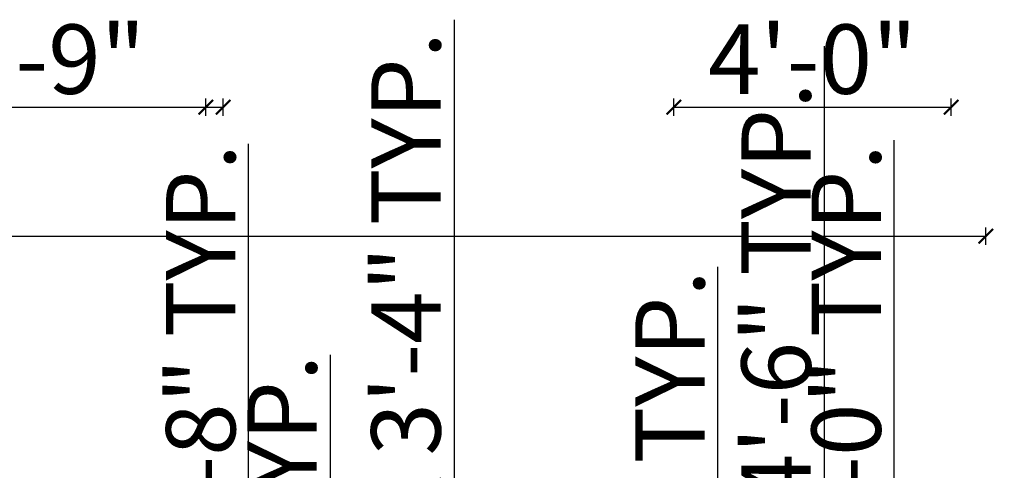
# Model space of a CAD drawing. Units: inches. Extents: x 375 to 1122, y 27 to 1069.
# Tile 154 of 155: x 819 to 989, y 991 to 1069. Entities that reach past the tile are written whole.
import ezdxf

# ---------------------------------------------------------------- set-up
doc = ezdxf.new("R2010")
doc.units = ezdxf.units.IN
doc.layers.add('A-ANNO-DIMS', color=2, linetype='Continuous', lineweight=18)
doc.styles.get("Standard").update_dxf_attribs({"font": 'arial.ttf'})
doc.dimstyles.new('ISO-25', dxfattribs={"dimtxt": 12, "dimasz": 2.5, "dimexe": 1.5, "dimexo": 1.5, "dimtad": 1, "dimdec": 1, "dimlunit": 3, "dimtxsty": 'Standard', "dimblk": 'ARCHTICK', "dimcen": 2.5, "dimadec": 0, "dimazin": 0, "dimtfac": 1, "dimtdec": 1, "dimtmove": 0, "dimatfit": 3, "dimfxl": 1.5, "dimfxlon": 1, "dimarcsym": 0})

# ---------------------------------------------------------------- blocks, each defined once
blk = doc.blocks.new('_ArchTick')
at = {"color": 0, "linetype": 'ByBlock', "const_width": 0.15}
blk.add_lwpolyline([(-0.5, -0.5), (0.5, 0.5)], dxfattribs=at)
blk = doc.blocks.new('*D27')
at = {"layer": 'A-ANNO-DIMS', "color": 0, "lineweight": -2, "transparency": 16777216}
for p, q in [((444.51, 1030.21), (444.51, 1033.21)), ((986.01, 1030.21), (986.01, 1033.21)), ((444.51, 1031.71), (986.01, 1031.71))]:
    blk.add_line(p, q, dxfattribs=at)
at = {"layer": 'Defpoints', "color": 0, "transparency": 16777216}
for p in [(986.01, 1031.71), (444.51, 982.53), (986.01, 982.53)]:
    blk.add_point(p, dxfattribs=at)
at = {"layer": 'A-ANNO-DIMS', "color": 0, "lineweight": -2, "transparency": 16777216, "xscale": 2.5, "yscale": 2.5, "zscale": 2.5, "rotation": 180}
blk.add_blockref('_ArchTick', (444.51, 1031.71), dxfattribs=at)
at = {"layer": 'A-ANNO-DIMS', "color": 0, "lineweight": -2, "transparency": 16777216, "xscale": 2.5, "yscale": 2.5, "zscale": 2.5}
blk.add_blockref('_ArchTick', (986.01, 1031.71), dxfattribs=at)
at = {"layer": 'A-ANNO-DIMS', "color": 0, "transparency": 16777216, "insert": (715.26, 1038.46), "char_height": 12, "attachment_point": 5}
blk.add_mtext('45\'-1.5"', dxfattribs=at)
blk = doc.blocks.new('*D62')
at = {"layer": 'A-ANNO-DIMS', "color": 0, "lineweight": -2, "transparency": 16777216}
for p, q in [((872.61, 898.16), (872.61, 1011.21)), ((871.11, 898.16), (874.11, 898.16)), ((872.61, 874.53), (872.61, 898.16)), ((871.11, 874.53), (874.11, 874.53))]:
    blk.add_line(p, q, dxfattribs=at)
at = {"layer": 'Defpoints', "color": 0, "transparency": 16777216}
for p in [(869.01, 898.16), (872.61, 898.16), (869.01, 874.53)]:
    blk.add_point(p, dxfattribs=at)
at = {"layer": 'A-ANNO-DIMS', "color": 0, "lineweight": -2, "transparency": 16777216, "xscale": 2.5, "yscale": 2.5, "zscale": 2.5}
for p, rotation in [((872.61, 898.16), 90), ((872.61, 874.53), 270)]:
    blk.add_blockref('_ArchTick', p, dxfattribs=dict(at, rotation=rotation))
at = {"layer": 'A-ANNO-DIMS', "color": 0, "transparency": 16777216, "insert": (865.78, 955.93), "char_height": 12, "attachment_point": 5, "rotation": 90}
blk.add_mtext('1\'-11 1/2" TYP.', dxfattribs=at)
blk = doc.blocks.new('*D63')
at = {"layer": 'A-ANNO-DIMS', "color": 0, "lineweight": -2, "transparency": 16777216}
for p, q in [((894.04, 948.53), (894.04, 1069.15)), ((895.54, 948.53), (892.54, 948.53)), ((894.04, 908.53), (894.04, 948.53)), ((895.54, 908.53), (892.54, 908.53))]:
    blk.add_line(p, q, dxfattribs=at)
at = {"layer": 'Defpoints', "color": 0, "transparency": 16777216}
for p in [(894.04, 948.53), (900.04, 948.53), (900.04, 908.53)]:
    blk.add_point(p, dxfattribs=at)
at = {"layer": 'A-ANNO-DIMS', "color": 0, "lineweight": -2, "transparency": 16777216, "xscale": 2.5, "yscale": 2.5, "zscale": 2.5}
for p, rotation in [((894.04, 948.53), 90), ((894.04, 908.53), 270)]:
    blk.add_blockref('_ArchTick', p, dxfattribs=dict(at, rotation=rotation))
at = {"layer": 'A-ANNO-DIMS', "color": 0, "transparency": 16777216, "insert": (887.21, 1010.09), "char_height": 12, "attachment_point": 5, "rotation": 90}
blk.add_mtext('SINK 3\'-4" TYP.', dxfattribs=at)
blk = doc.blocks.new('*D66')
at = {"layer": 'A-ANNO-DIMS', "color": 0, "lineweight": -2, "transparency": 16777216}
for p, q in [((970.15, 971.21), (970.15, 1048.31)), ((968.65, 971.21), (971.65, 971.21)), ((970.15, 947.21), (970.15, 971.21)), ((968.65, 947.21), (971.65, 947.21))]:
    blk.add_line(p, q, dxfattribs=at)
at = {"layer": 'Defpoints', "color": 0, "transparency": 16777216}
for p in [(966.55, 971.21), (970.15, 971.21), (966.55, 947.21)]:
    blk.add_point(p, dxfattribs=at)
at = {"layer": 'A-ANNO-DIMS', "color": 0, "lineweight": -2, "transparency": 16777216, "xscale": 2.5, "yscale": 2.5, "zscale": 2.5}
for p, rotation in [((970.15, 971.21), 90), ((970.15, 947.21), 270)]:
    blk.add_blockref('_ArchTick', p, dxfattribs=dict(at, rotation=rotation))
at = {"layer": 'A-ANNO-DIMS', "color": 0, "transparency": 16777216, "insert": (963.4, 1011.01), "char_height": 12, "attachment_point": 5, "rotation": 90}
blk.add_mtext('2\'-0" TYP.', dxfattribs=at)
blk = doc.blocks.new('*D68')
at = {"layer": 'A-ANNO-DIMS', "color": 0, "lineweight": -2, "transparency": 16777216}
for p, q in [((858.44, 971.91), (858.44, 1047.67)), ((856.94, 971.91), (859.94, 971.91)), ((858.44, 951.91), (858.44, 971.91)), ((856.94, 951.91), (859.94, 951.91))]:
    blk.add_line(p, q, dxfattribs=at)
at = {"layer": 'Defpoints', "color": 0, "transparency": 16777216}
for p in [(853.33, 971.91), (858.44, 971.91), (853.33, 951.91)]:
    blk.add_point(p, dxfattribs=at)
at = {"layer": 'A-ANNO-DIMS', "color": 0, "lineweight": -2, "transparency": 16777216, "xscale": 2.5, "yscale": 2.5, "zscale": 2.5}
for p, rotation in [((858.44, 971.91), 90), ((858.44, 951.91), 270)]:
    blk.add_blockref('_ArchTick', p, dxfattribs=dict(at, rotation=rotation))
at = {"layer": 'A-ANNO-DIMS', "color": 0, "transparency": 16777216, "insert": (851.69, 1011.04), "char_height": 12, "attachment_point": 5, "rotation": 90}
blk.add_mtext('1\'-8" TYP.', dxfattribs=at)
blk = doc.blocks.new('*D75')
at = {"layer": 'A-ANNO-DIMS', "color": 0, "lineweight": -2, "transparency": 16777216}
for p, q in [((958.11, 868.53), (958.11, 1064.59)), ((956.61, 868.53), (959.61, 868.53)), ((958.11, 814.53), (958.11, 868.53)), ((956.61, 814.53), (959.61, 814.53))]:
    blk.add_line(p, q, dxfattribs=at)
at = {"layer": 'Defpoints', "color": 0, "transparency": 16777216}
for p in [(950.01, 868.53), (958.11, 868.53), (950.01, 814.53)]:
    blk.add_point(p, dxfattribs=at)
at = {"layer": 'A-ANNO-DIMS', "color": 0, "lineweight": -2, "transparency": 16777216, "xscale": 2.5, "yscale": 2.5, "zscale": 2.5}
for p, rotation in [((958.11, 868.53), 90), ((958.11, 814.53), 270)]:
    blk.add_blockref('_ArchTick', p, dxfattribs=dict(at, rotation=rotation))
at = {"layer": 'A-ANNO-DIMS', "color": 0, "transparency": 16777216, "insert": (951.27, 967.81), "char_height": 12, "attachment_point": 5, "rotation": 90}
blk.add_mtext('SHOWER PAN 4\'-6" TYP.', dxfattribs=at)
blk = doc.blocks.new('*D78')
at = {"layer": 'A-ANNO-DIMS', "color": 0, "lineweight": -2, "transparency": 16777216}
for p, q in [((939.66, 949.53), (939.66, 1026.42)), ((938.16, 949.53), (941.16, 949.53)), ((939.66, 907.53), (939.66, 949.53)), ((938.16, 907.53), (941.16, 907.53))]:
    blk.add_line(p, q, dxfattribs=at)
at = {"layer": 'Defpoints', "color": 0, "transparency": 16777216}
for p in [(923.01, 949.53), (939.66, 949.53), (923.01, 907.53)]:
    blk.add_point(p, dxfattribs=at)
at = {"layer": 'A-ANNO-DIMS', "color": 0, "lineweight": -2, "transparency": 16777216, "xscale": 2.5, "yscale": 2.5, "zscale": 2.5}
for p, rotation in [((939.66, 949.53), 90), ((939.66, 907.53), 270)]:
    blk.add_blockref('_ArchTick', p, dxfattribs=dict(at, rotation=rotation))
at = {"layer": 'A-ANNO-DIMS', "color": 0, "transparency": 16777216, "insert": (932.9, 989.22), "char_height": 12, "attachment_point": 5, "rotation": 90}
blk.add_mtext('3\'-6" TYP.', dxfattribs=at)
blk = doc.blocks.new('*D83')
at = {"layer": 'A-ANNO-DIMS', "color": 0, "lineweight": -2, "transparency": 16777216}
for p, q in [((932.01, 1052.53), (932.01, 1055.53)), ((980.01, 1052.53), (980.01, 1055.53)), ((932.01, 1054.03), (980.01, 1054.03))]:
    blk.add_line(p, q, dxfattribs=at)
at = {"layer": 'Defpoints', "color": 0, "transparency": 16777216}
for p in [(980.01, 1054.03), (932.01, 973.53), (980.01, 973.53)]:
    blk.add_point(p, dxfattribs=at)
at = {"layer": 'A-ANNO-DIMS', "color": 0, "lineweight": -2, "transparency": 16777216, "xscale": 2.5, "yscale": 2.5, "zscale": 2.5, "rotation": 180}
blk.add_blockref('_ArchTick', (932.01, 1054.03), dxfattribs=at)
at = {"layer": 'A-ANNO-DIMS', "color": 0, "lineweight": -2, "transparency": 16777216, "xscale": 2.5, "yscale": 2.5, "zscale": 2.5}
blk.add_blockref('_ArchTick', (980.01, 1054.03), dxfattribs=at)
at = {"layer": 'A-ANNO-DIMS', "color": 0, "transparency": 16777216, "insert": (956.01, 1060.78), "char_height": 12, "attachment_point": 5}
blk.add_mtext('4\'-0"', dxfattribs=at)
blk = doc.blocks.new('*D88')
at = {"layer": 'A-ANNO-DIMS', "color": 0, "lineweight": -2, "transparency": 16777216}
for p, q in [((731.01, 1052.53), (731.01, 1055.53)), ((854.01, 1052.53), (854.01, 1055.53)), ((731.01, 1054.03), (854.01, 1054.03))]:
    blk.add_line(p, q, dxfattribs=at)
at = {"layer": 'Defpoints', "color": 0, "transparency": 16777216}
for p in [(854.01, 1054.03), (731.01, 502.53), (854.01, 502.53)]:
    blk.add_point(p, dxfattribs=at)
at = {"layer": 'A-ANNO-DIMS', "color": 0, "lineweight": -2, "transparency": 16777216, "xscale": 2.5, "yscale": 2.5, "zscale": 2.5, "rotation": 180}
blk.add_blockref('_ArchTick', (731.01, 1054.03), dxfattribs=at)
at = {"layer": 'A-ANNO-DIMS', "color": 0, "lineweight": -2, "transparency": 16777216, "xscale": 2.5, "yscale": 2.5, "zscale": 2.5}
blk.add_blockref('_ArchTick', (854.01, 1054.03), dxfattribs=at)
at = {"layer": 'A-ANNO-DIMS', "color": 0, "transparency": 16777216, "insert": (792.51, 1060.78), "char_height": 12, "attachment_point": 5}
blk.add_mtext('10\'-3"', dxfattribs=at)
blk = doc.blocks.new('*D96')
at = {"layer": 'A-ANNO-DIMS', "color": 0, "lineweight": -2, "transparency": 16777216}
for p, q in [((794.01, 1052.53), (794.01, 1055.53)), ((851.01, 1052.53), (851.01, 1055.53)), ((794.01, 1054.03), (851.01, 1054.03))]:
    blk.add_line(p, q, dxfattribs=at)
at = {"layer": 'Defpoints', "color": 0, "transparency": 16777216}
for p in [(851.01, 1054.03), (794.01, 973.53), (851.01, 973.53)]:
    blk.add_point(p, dxfattribs=at)
at = {"layer": 'A-ANNO-DIMS', "color": 0, "lineweight": -2, "transparency": 16777216, "xscale": 2.5, "yscale": 2.5, "zscale": 2.5, "rotation": 180}
blk.add_blockref('_ArchTick', (794.01, 1054.03), dxfattribs=at)
at = {"layer": 'A-ANNO-DIMS', "color": 0, "lineweight": -2, "transparency": 16777216, "xscale": 2.5, "yscale": 2.5, "zscale": 2.5}
blk.add_blockref('_ArchTick', (851.01, 1054.03), dxfattribs=at)
at = {"layer": 'A-ANNO-DIMS', "color": 0, "transparency": 16777216, "insert": (822.51, 1060.78), "char_height": 12, "attachment_point": 5}
blk.add_mtext('4\'-9"', dxfattribs=at)

msp = doc.modelspace()

# ---------------------------------------------------------------- dimensions: what is measured, and where the dimension line sits
at = {"layer": 'A-ANNO-DIMS'}
for base, p1, p2, picture, middle in [((854.01, 1054.03), (731.01, 502.53), (854.01, 502.53), '*D88', (792.51, 1060.78)), ((851.01, 1054.03), (794.01, 973.53), (851.01, 973.53), '*D96', (822.51, 1060.78)), ((980.01, 1054.03), (932.01, 973.53), (980.01, 973.53), '*D83', (956.01, 1060.78))]:
    dim = msp.add_linear_dim(base=base, p1=p1, p2=p2, dimstyle='ISO-25', override={"dimdec": 1, "dimlfac": 1, "dimrnd": 0, "dimzin": 1, "dimdsep": 46, "dimlunit": 4, "dimfrac": 2}, dxfattribs=at)
    dim.commit()
    dim.dimension.update_dxf_attribs({"geometry": picture, "text_midpoint": middle})
for base, p1, p2, text, picture, middle in [((894.04, 948.53), (900.04, 908.53), (900.04, 948.53), 'SINK <> TYP.', '*D63', (887.21, 1010.09)), ((958.11, 868.53), (950.01, 814.53), (950.01, 868.53), 'SHOWER PAN <> TYP.', '*D75', (951.27, 967.81)), ((970.15, 971.21), (966.55, 947.21), (966.55, 971.21), '<> TYP.', '*D66', (963.4, 1011.01)), ((858.44, 971.91), (853.33, 951.91), (853.33, 971.91), '<> TYP.', '*D68', (851.69, 1011.04)), ((939.66, 949.53), (923.01, 907.53), (923.01, 949.53), '<> TYP.', '*D78', (932.9, 989.22)), ((872.61, 898.16), (869.01, 874.53), (869.01, 898.16), '<> TYP.', '*D62', (865.78, 955.93))]:
    dim = msp.add_linear_dim(base=base, p1=p1, p2=p2, angle=90, text=text, dimstyle='ISO-25', override={"dimdec": 1, "dimlfac": 1, "dimrnd": 0, "dimzin": 1, "dimdsep": 46, "dimlunit": 4, "dimfrac": 2}, dxfattribs=at)
    dim.commit()
    dim.dimension.update_dxf_attribs({"geometry": picture, "text_midpoint": middle})
dim = msp.add_linear_dim(base=(986.01, 1031.71), p1=(444.51, 982.53), p2=(986.01, 982.53), dimstyle='ISO-25', override={"dimclrd": 0, "dimclre": 0, "dimclrt": 0}, dxfattribs=at)
dim.commit()
dim.dimension.update_dxf_attribs({"geometry": '*D27', "text_midpoint": (715.26, 1031.71), "dimtype": 160})

doc.saveas('drawing.dxf')
